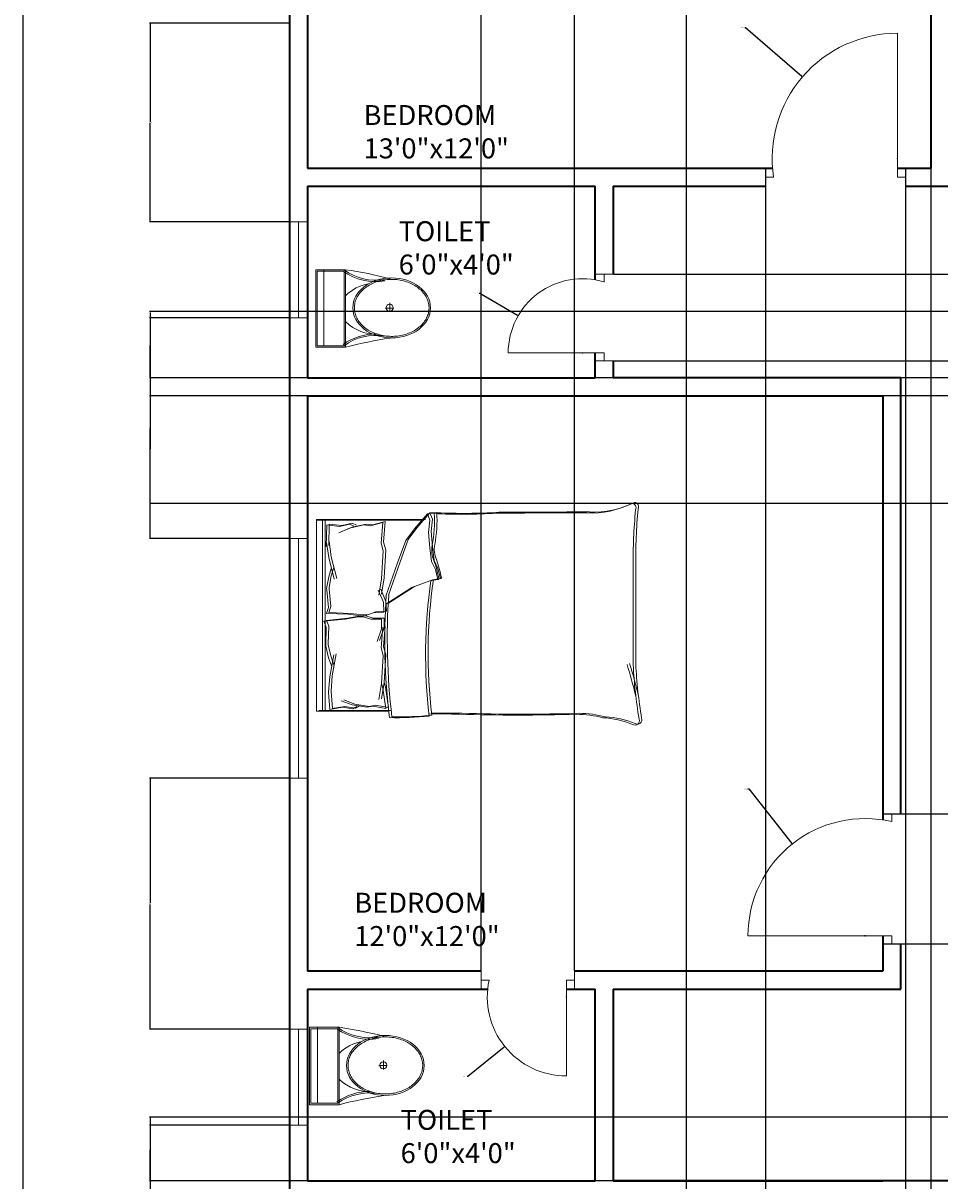
# Model space of a CAD drawing. Units: inches. Extents: x 1861 to 2564, y 1482 to 2317.
# Tile 4 of 11: x 1861 to 2090, y 1853 to 2143. Entities that reach past the tile are written whole.
import ezdxf

# ---------------------------------------------------------------- set-up
doc = ezdxf.new("R2010")
doc.units = ezdxf.units.IN
for name, color, linetype, lineweight in [('A-ANNO-DIMS', 2, 'Continuous', 18), ('A-ANNO-TTLB', 7, 'Continuous', 25), ('A-AREA-IDEN', 7, 'Continuous', 18), ('A-DOOR', 3, 'Continuous', 18), ('A-FLOR-FIXT', 8, 'Continuous', 18), ('A-FURN', 8, 'Continuous', 13), ('A-GLAZ', 4, 'Continuous', 18), ('A-WALL', 7, 'Continuous', 35)]:
    doc.layers.add(name, color=color, linetype=linetype, lineweight=lineweight)
doc.styles.get("Standard").update_dxf_attribs({"font": 'arial.ttf'})
doc.dimstyles.get("Standard").update_dxf_attribs({"dimtxt": 0.18, "dimasz": 0.18, "dimexe": 0.18, "dimexo": 0.0625, "dimgap": 0.09, "dimtad": 0, "dimtih": 1, "dimtoh": 1, "dimdec": 4, "dimzin": 0, "dimdsep": 46, "dimtxsty": 'Standard', "dimcen": 0.09, "dimadec": 0, "dimazin": 0, "dimtfac": 1, "dimtdec": 4, "dimtofl": 0, "dimtmove": 0, "dimatfit": 3, "dimfxl": 1, "dimtolj": 1, "dimtzin": 0, "dimarcsym": 0})

# ---------------------------------------------------------------- blocks, each defined once
blk = doc.blocks.new('A$C31115884')
for p, q in [((283.1, 497.7), (223.4, 497.7)), ((257.5, 466.4), (257.5, 523.2)), ((0, 200), (0, 0)), ((520, 200), (0, 200)), ((10, 190), (10, 10)), ((510, 190), (10, 190)), ((510, 10), (510, 190)), ((520, 0), (520, 200)), ((510, 54.5), (0, 54.5)), ((10, 10), (510, 10)), ((0, 0), (520, 0))]:
    blk.add_line(p, q)
blk.add_circle((255.6, 496.4), 23.6)
for centre, radius, start, end in [((2777.7, -204.6), 2807, 165.4549, 171.71327), ((3237, 905), 2807, 188.28673, 194.5451), ((-294.5, 403.3), 364.7, 324.20913, 9.34987), ((-294.5, 403.3), 374.7, 324.20913, 9.34987), ((139.5, 406.2), 293.5, 315.84364, 2.65635), ((805.8, 403.3), 374.7, 179.20365, 215.79087), ((805.8, 403.3), 364.7, 170.65013, 215.79087), ((383.6, 406.2), 293.5, 190.27735, 224.15636)]:
    blk.add_arc(centre, radius, start, end)
blk.add_ellipse((256.2, 509.9), major_axis=(0, -260.7), ratio=0.772727)
blk.add_open_spline([(256.2, 259.2), (263.1, 259.2), (270, 259.7), (287.8, 262.3), (298.7, 265.1), (319.9, 273.1), (330.2, 278.4), (350.1, 291.1), (359.7, 298.7), (377.7, 315.9), (386.2, 325.5), (401.7, 346.6), (408.8, 358.1), (421.3, 382.5), (426.8, 395.5), (435.9, 422.4), (439.5, 436.4), (444.8, 465.1), (446.5, 479.7), (447.9, 509.2), (447.6, 524), (445, 553.3), (442.7, 567.8), (436.3, 596), (432.1, 609.7), (421.9, 636), (416, 648.6), (402.5, 672.1), (395, 683), (378.6, 703), (369.8, 712.1), (351.1, 728), (341.3, 734.8), (320.9, 746.2), (310.4, 750.7), (288.9, 757.3), (278, 759.4), (256, 761), (245, 760.6), (223.1, 757.2), (212.3, 754.3), (191.1, 746.1), (180.8, 740.7), (160.9, 727.8), (151.4, 720.1), (133.5, 702.7), (125.1, 693), (109.6, 671.7), (102.6, 660.2), (90.2, 635.7), (84.9, 622.7), (76, 595.6), (72.4, 581.6), (67.2, 552.9), (65.6, 538.2), (64.4, 508.8), (64.8, 494), (67.5, 464.7), (69.9, 450.2), (76.6, 422), (80.8, 408.3), (91.1, 382.2), (97.2, 369.7), (110.8, 346.3), (118.4, 335.4), (134.8, 315.6), (143.7, 306.7), (162.4, 290.9), (172.3, 284.2), (192.8, 273), (203.3, 268.6), (224.8, 262.2), (235.8, 260.2), (249.9, 259.3), (253, 259.2), (256.2, 259.2)], degree=3, knots=[0, 0, 0, 0, 0.110105, 0.110105, 0.285049, 0.285049, 0.459994, 0.459994, 0.634938, 0.634938, 0.809882, 0.809882, 0.984827, 0.984827, 1.159771, 1.159771, 1.334715, 1.334715, 1.50966, 1.50966, 1.684604, 1.684604, 1.859549, 1.859549, 2.034493, 2.034493, 2.209437, 2.209437, 2.384382, 2.384382, 2.559326, 2.559326, 2.73427, 2.73427, 2.909215, 2.909215, 3.084159, 3.084159, 3.259103, 3.259103, 3.434048, 3.434048, 3.608992, 3.608992, 3.783936, 3.783936, 3.958881, 3.958881, 4.133825, 4.133825, 4.30877, 4.30877, 4.483714, 4.483714, 4.658658, 4.658658, 4.833603, 4.833603, 5.008547, 5.008547, 5.183491, 5.183491, 5.358436, 5.358436, 5.53338, 5.53338, 5.708324, 5.708324, 5.883269, 5.883269, 6.058213, 6.058213, 6.233158, 6.233158, 6.283185, 6.283185, 6.283185, 6.283185])
blk = doc.blocks.new('WIN-24IN')
for p, q in [((0, 24), (4.5, 24)), ((4.5, 24), (2.25, 24)), ((2.25, 24), (2.25, 0)), ((2.25, 0), (0, 0)), ((0, 0), (4.5, 0))]:
    blk.add_line(p, q)
blk = doc.blocks.new('BED-DOUBLE')
for p, q in [((3.48, 63.34), (3.48, 81.45)), ((3.48, 63.34), (3.48, 81.45)), ((51.27, 81.45), (3.48, 81.45)), ((51.27, 81.45), (51.27, 54.84)), ((51.27, 81.45), (51.27, 54.84)), ((51.27, 81.45), (51.49, 81.45)), ((51.49, 81.45), (51.49, 80.81)), ((3.48, 79.91), (51.27, 79.91)), ((3.48, 79.91), (51.27, 79.91)), ((3.7, 62.7), (3.7, 80.81)), ((3.7, 62.7), (3.7, 80.81)), ((3.7, 79.27), (51.49, 79.27)), ((3.7, 79.27), (51.49, 79.27)), ((3.9, 78.11), (8.18, 78.44)), ((3.9, 78.11), (8.18, 78.44)), ((8.18, 78.44), (8.29, 78.42)), ((8.18, 78.44), (8.29, 78.42)), ((8.29, 78.42), (12.11, 78.13)), ((8.29, 78.42), (12.11, 78.13)), ((14.86, 77.7), (16.88, 78.42)), ((14.86, 77.7), (16.88, 78.42)), ((16.88, 78.42), (19.77, 79.14)), ((16.88, 78.42), (19.77, 79.14)), ((17.11, 77.78), (20, 78.5)), ((17.11, 77.78), (20, 78.5)), ((19.77, 79.14), (20.09, 79.14)), ((19.77, 79.14), (20.09, 79.14)), ((20, 78.5), (20.32, 78.5)), ((20, 78.5), (20.32, 78.5)), ((20.09, 79.14), (24.54, 79)), ((20.09, 79.14), (24.54, 79)), ((20.32, 78.5), (24.77, 78.36)), ((20.32, 78.5), (24.77, 78.36)), ((24.54, 79), (25.98, 79.58)), ((24.54, 79), (25.98, 79.58)), ((24.77, 78.36), (26.21, 78.94)), ((24.77, 78.36), (26.21, 78.94)), ((25.98, 79.58), (26.56, 74.23)), ((25.98, 79.58), (26.56, 74.23)), ((26.21, 78.94), (26.79, 73.59)), ((26.21, 78.94), (26.79, 73.59)), ((27.98, 78.95), (27.73, 73.58)), ((27.98, 78.95), (27.73, 73.58)), ((28.21, 78.31), (27.96, 72.94)), ((28.21, 78.31), (27.96, 72.94)), ((29.46, 78.47), (27.98, 78.95)), ((29.46, 78.47), (27.98, 78.95)), ((29.69, 77.83), (28.21, 78.31)), ((29.68, 77.83), (28.21, 78.31)), ((33.88, 78.89), (29.46, 78.47)), ((33.88, 78.89), (29.46, 78.47)), ((34.11, 78.25), (29.68, 77.83)), ((34.11, 78.25), (29.69, 77.83)), ((34.21, 78.91), (33.88, 78.89)), ((34.21, 78.91), (33.88, 78.89)), ((34.43, 78.27), (34.11, 78.25)), ((34.43, 78.27), (34.11, 78.25)), ((37.14, 78.37), (34.21, 78.91)), ((37.14, 78.37), (34.21, 78.91)), ((37.36, 77.73), (34.43, 78.27)), ((37.36, 77.73), (34.43, 78.27)), ((41.92, 78.38), (36.5, 77.02)), ((41.92, 78.38), (36.5, 77.02)), ((39.2, 77.77), (37.14, 78.37)), ((39.2, 77.77), (37.14, 78.37)), ((45.71, 78.9), (41.92, 78.38)), ((45.71, 78.9), (41.92, 78.38)), ((45.94, 78.26), (42.14, 77.74)), ((45.94, 78.26), (42.14, 77.74)), ((50.11, 78.89), (44.71, 78.99)), ((44.71, 78.99), (45.71, 78.9)), ((50.11, 78.89), (44.71, 78.99)), ((44.71, 78.99), (45.71, 78.9)), ((50.34, 78.25), (44.94, 78.35)), ((44.94, 78.35), (45.94, 78.26)), ((50.34, 78.25), (44.94, 78.35)), ((44.94, 78.35), (45.94, 78.26)), ((50.11, 78.89), (49.73, 75.68)), ((50.11, 78.89), (49.73, 75.68)), ((50.34, 78.25), (49.96, 75.04)), ((50.34, 78.25), (49.96, 75.04)), ((51.49, 80.81), (51.49, 54.2)), ((51.49, 80.81), (51.49, 54.2)), ((3.9, 78.13), (4.47, 74.95)), ((3.9, 78.13), (4.47, 74.95)), ((4.12, 77.49), (4.7, 74.31)), ((4.12, 77.49), (4.7, 74.31)), ((4.13, 77.47), (8.41, 77.8)), ((4.13, 77.47), (8.41, 77.8)), ((8.41, 77.8), (8.51, 77.78)), ((8.41, 77.8), (8.51, 77.78)), ((8.51, 77.78), (12.34, 77.49)), ((8.51, 77.78), (12.34, 77.49)), ((12.11, 78.13), (17.6, 77.12)), ((12.11, 78.13), (17.6, 77.12)), ((12.34, 77.49), (17.83, 76.48)), ((12.34, 77.49), (17.83, 76.48)), ((15.08, 77.06), (17.11, 77.78)), ((15.08, 77.06), (17.11, 77.78)), ((42.14, 77.74), (36.72, 76.38)), ((42.14, 77.74), (36.72, 76.38)), ((39.43, 77.13), (37.36, 77.73)), ((39.43, 77.13), (37.36, 77.73)), ((49.31, 73.19), (48.13, 75.87)), ((49.31, 73.19), (48.13, 75.87)), ((49.73, 75.68), (50.33, 73.11)), ((49.73, 75.68), (50.33, 73.11)), ((4.47, 74.95), (4.04, 72.35)), ((4.47, 74.95), (4.04, 72.35)), ((4.7, 74.31), (4.27, 71.71)), ((4.7, 74.31), (4.27, 71.71)), ((4.47, 68.88), (5.05, 72.49)), ((4.47, 68.88), (5.05, 72.49)), ((5.05, 72.49), (6.06, 75.24)), ((5.05, 72.49), (6.06, 75.24)), ((5.28, 71.85), (6.29, 74.6)), ((5.28, 71.85), (6.29, 74.6)), ((26.56, 74.23), (27.14, 71.04)), ((26.56, 74.23), (27.14, 71.04)), ((26.79, 73.59), (27.37, 70.41)), ((26.79, 73.59), (27.37, 70.41)), ((27.73, 73.58), (27.36, 70.37)), ((27.73, 73.58), (27.36, 70.37)), ((27.96, 72.94), (27.58, 69.73)), ((27.96, 72.94), (27.58, 69.73)), ((49.54, 72.55), (48.36, 75.23)), ((49.54, 72.55), (48.36, 75.23)), ((50.11, 69.62), (49.31, 73.19)), ((50.11, 69.62), (49.31, 73.19)), ((50.34, 68.98), (49.54, 72.55)), ((50.34, 68.98), (49.54, 72.55)), ((50.33, 73.11), (49.82, 72.06)), ((50.33, 73.11), (49.82, 72.06)), ((49.96, 75.04), (50.56, 72.47)), ((49.96, 75.04), (50.56, 72.47)), ((50.56, 72.47), (50.04, 71.42)), ((50.56, 72.47), (50.04, 71.42)), ((4.04, 72.35), (4.62, 71.33)), ((4.04, 72.35), (4.62, 71.33)), ((4.27, 71.71), (4.85, 70.69)), ((4.27, 71.71), (4.85, 70.69)), ((4.7, 68.24), (5.28, 71.85)), ((4.7, 68.24), (5.28, 71.85)), ((27.14, 69.74), (26.56, 67.86)), ((27.14, 69.74), (26.56, 67.86)), ((27.14, 71.04), (27.14, 69.74)), ((27.14, 71.04), (27.14, 69.74)), ((27.36, 70.37), (27.44, 69.07)), ((27.36, 70.37), (27.44, 69.07)), ((27.37, 70.41), (27.37, 69.1)), ((27.37, 70.41), (27.37, 69.1)), ((27.58, 69.73), (27.67, 68.43)), ((27.58, 69.73), (27.67, 68.43)), ((49.92, 68.01), (50.11, 69.62)), ((49.92, 68.01), (50.11, 69.62)), ((4.18, 64.1), (4.76, 67.29)), ((4.18, 64.1), (4.76, 67.29)), ((4.76, 67.29), (4.47, 68.88)), ((4.76, 67.29), (4.47, 68.88)), ((4.99, 66.65), (4.7, 68.24)), ((4.99, 66.65), (4.7, 68.24)), ((26.56, 67.86), (26.56, 65.18)), ((26.56, 67.86), (26.56, 65.18)), ((27.37, 69.1), (26.79, 67.22)), ((27.37, 69.1), (26.79, 67.22)), ((26.79, 67.22), (26.79, 64.54)), ((26.79, 67.22), (26.79, 64.54)), ((27.44, 69.07), (28.13, 67.23)), ((27.44, 69.07), (28.13, 67.23)), ((27.67, 68.43), (28.36, 66.59)), ((27.67, 68.43), (28.36, 66.59)), ((28.13, 67.23), (28.3, 64.55)), ((28.13, 67.23), (28.3, 64.55)), ((50.7, 64.87), (49.92, 68.01)), ((50.7, 64.87), (49.92, 68.01)), ((50.15, 67.37), (50.34, 68.98)), ((50.15, 67.37), (50.34, 68.98)), ((50.93, 64.23), (50.15, 67.37)), ((50.93, 64.23), (50.15, 67.37)), ((9.28, 64.83), (4.18, 64.1)), ((9.28, 64.83), (4.18, 64.1)), ((4.41, 63.46), (4.99, 66.65)), ((4.41, 63.46), (4.99, 66.65)), ((9.51, 64.19), (4.41, 63.46)), ((9.51, 64.19), (4.41, 63.46)), ((6.38, 65.82), (10.41, 65.15)), ((6.38, 65.82), (10.41, 65.15)), ((6.61, 65.18), (10.64, 64.51)), ((6.61, 65.18), (10.64, 64.51)), ((10.41, 65.15), (9.28, 64.83)), ((10.41, 65.15), (9.28, 64.83)), ((10.64, 64.51), (9.51, 64.19)), ((10.64, 64.51), (9.51, 64.19)), ((10.41, 65.15), (17.42, 64.72)), ((10.41, 65.15), (17.42, 64.72)), ((10.64, 64.51), (17.65, 64.08)), ((10.64, 64.51), (17.65, 64.08)), ((17.42, 64.72), (19.38, 65.28)), ((17.42, 64.72), (19.38, 65.28)), ((17.65, 64.08), (19.61, 64.64)), ((17.65, 64.08), (19.61, 64.64)), ((19.38, 65.28), (24.52, 64.87)), ((19.38, 65.28), (24.52, 64.87)), ((19.61, 64.64), (24.75, 64.23)), ((19.61, 64.64), (24.74, 64.23)), ((24.1, 65.18), (20.96, 66.27)), ((24.1, 65.18), (20.96, 66.27)), ((24.33, 64.54), (21.19, 65.63)), ((24.33, 64.54), (21.19, 65.63)), ((26.56, 65.18), (24.1, 65.18)), ((26.56, 65.18), (24.1, 65.18)), ((26.79, 64.54), (24.33, 64.54)), ((26.79, 64.54), (24.33, 64.54)), ((28.3, 64.55), (30.75, 64.71)), ((28.3, 64.55), (30.75, 64.71)), ((28.36, 66.59), (28.53, 63.91)), ((28.36, 66.59), (28.53, 63.91)), ((28.53, 63.91), (30.98, 64.07)), ((28.53, 63.91), (30.98, 64.07)), ((30.26, 64.06), (34.45, 57.57)), ((30.26, 64.06), (34.45, 57.57)), ((30.75, 64.71), (33.82, 65.99)), ((30.75, 64.71), (33.82, 65.99)), ((30.98, 64.07), (34.05, 65.35)), ((30.98, 64.07), (34.05, 65.35)), ((40.65, 61.13), (32.31, 64.06)), ((40.64, 61.13), (32.31, 64.06)), ((32.56, 65.82), (36.6, 65.15)), ((32.57, 65.82), (36.6, 65.15)), ((32.79, 65.18), (36.83, 64.51)), ((32.79, 65.18), (36.83, 64.51)), ((36.6, 65.15), (43.61, 64.72)), ((36.6, 65.15), (43.61, 64.72)), ((36.83, 64.51), (43.84, 64.08)), ((36.83, 64.51), (43.84, 64.08)), ((43.61, 64.72), (45.57, 65.28)), ((43.61, 64.72), (45.57, 65.28)), ((43.84, 64.08), (45.8, 64.64)), ((43.84, 64.08), (45.8, 64.64)), ((45.57, 65.28), (50.7, 64.87)), ((45.57, 65.28), (50.7, 64.87)), ((45.8, 64.64), (50.93, 64.23)), ((45.8, 64.64), (50.93, 64.23)), ((30.49, 63.42), (34.68, 56.93)), ((30.49, 63.42), (34.68, 56.93)), ((40.87, 60.49), (32.54, 63.42)), ((40.87, 60.49), (32.54, 63.42)), ((46.22, 59.12), (40.64, 61.13)), ((46.22, 59.12), (40.65, 61.13)), ((46.45, 58.48), (40.87, 60.49)), ((46.45, 58.48), (40.87, 60.49)), ((49.16, 56.95), (46.22, 59.12)), ((49.16, 56.95), (46.22, 59.12)), ((49.39, 56.31), (46.45, 58.48)), ((49.39, 56.31), (46.45, 58.48)), ((34.45, 57.57), (36.15, 53.08)), ((34.45, 57.57), (36.15, 53.08)), ((34.68, 56.93), (36.38, 52.44)), ((34.68, 56.93), (36.38, 52.44)), ((52.87, 53.7), (49.16, 56.95)), ((52.87, 53.7), (49.16, 56.95)), ((53.1, 53.06), (49.39, 56.31)), ((53.1, 53.06), (49.39, 56.31)), ((36.15, 53.08), (36.46, 51.07)), ((36.15, 53.08), (36.46, 51.07)), ((36.38, 52.44), (36.69, 50.43)), ((36.38, 52.44), (36.69, 50.43)), ((38.94, 51.69), (40.95, 52.62)), ((38.94, 51.69), (40.95, 52.62)), ((40.95, 52.62), (44.36, 53.08)), ((40.95, 52.62), (44.36, 53.08)), ((41.18, 51.98), (44.59, 52.44)), ((41.18, 51.98), (44.59, 52.44)), ((44.36, 53.08), (48.23, 53.39)), ((44.36, 53.08), (48.23, 53.39)), ((44.59, 52.44), (48.46, 52.75)), ((44.59, 52.44), (48.46, 52.75)), ((48.23, 53.39), (51.33, 53.08)), ((48.23, 53.39), (51.33, 53.08)), ((48.46, 52.75), (51.56, 52.44)), ((48.46, 52.75), (51.56, 52.44)), ((51.33, 53.08), (52.87, 53.7)), ((51.33, 53.08), (52.87, 53.7)), ((51.56, 52.44), (53.1, 53.06)), ((51.56, 52.44), (53.1, 53.06)), ((52.95, 51.95), (52.87, 53.7, 3.87)), ((52.95, 51.95), (52.87, 53.7, 3.87)), ((53.18, 51.32), (53.1, 53.06, 3.87)), ((53.18, 51.32), (53.1, 53.06, 3.87)), ((36.46, 51.07), (38.94, 51.69)), ((36.46, 51.07), (38.94, 51.69)), ((36.69, 50.43), (39.17, 51.05)), ((36.69, 50.43), (39.17, 51.05)), ((39.17, 51.05), (41.18, 51.98)), ((39.17, 51.05), (41.18, 51.98)), ((15.06, 2.2), (39.68, 2.2)), ((15.06, 2.2), (39.68, 2.2)), ((15.29, 1.56), (39.91, 1.56)), ((15.29, 1.56), (39.91, 1.56))]:
    blk.add_line(p, q)
for centre, radius, start, end in [((21.36, -100.61), 164.97, 86.0865, 96.7821), ((21.36, -100.61), 164.97, 86.0865, 96.7821), ((85.16, 61.35), 83.31, 178.7218, 185.604), ((85.16, 61.35), 83.31, 178.7218, 185.604), ((85.39, 60.71), 83.31, 178.7218, 185.604), ((85.39, 60.71), 83.31, 178.7218, 185.604), ((21.59, -101.25), 164.97, 86.0865, 96.7821), ((21.59, -101.25), 164.97, 86.0865, 96.7821), ((17.76, -74.87), 129.02, 81.7845, 96.9006), ((17.76, -74.87), 129.02, 81.7845, 96.9006), ((17.99, -75.51), 129.02, 81.7845, 96.9006), ((17.98, -75.51), 129.02, 81.7845, 96.9006), ((-167.31, 50.27), 170.11, 358.4762, 1.0082), ((-167.31, 50.27), 170.11, 358.4762, 1.0082), ((-167.08, 49.63), 170.11, 358.4762, 1.0082), ((-167.08, 49.63), 170.11, 358.4762, 1.0082), ((43.74, 46.38), 6.22, 78.6608, 113.7384), ((43.74, 46.38), 6.22, 78.6608, 113.7384), ((51.33, 88.1), 36.18, 259.8763, 272.5657), ((51.33, 88.1), 36.18, 259.8763, 272.5657), ((36.64, 51.01), 0.185, 160.2464, 271.1377), ((36.64, 51.01), 0.185, 160.2464, 271.1377), ((31.15, 79.96), 29.65, 280.6617, 289.8806), ((31.15, 79.96), 29.65, 280.6617, 289.8806), ((36.87, 50.37), 0.185, 160.2464, 271.1377), ((36.87, 50.37), 0.185, 160.2464, 271.1377), ((31.38, 79.32), 29.65, 280.6617, 289.8806), ((31.38, 79.32), 29.65, 280.6617, 289.8806), ((43.97, 45.74), 6.22, 78.6608, 113.7384), ((43.97, 45.74), 6.22, 78.6608, 113.7384), ((51.56, 87.46), 36.18, 259.8763, 272.5657), ((51.56, 87.46), 36.18, 259.8763, 272.5657), ((182.27, 45.13), 129.5, 176.9791, 183.8365), ((182.27, 45.13), 129.5, 176.9791, 183.8365), ((182.5, 44.49), 129.5, 176.9791, 183.8365), ((182.49, 44.49), 129.5, 176.9791, 183.8365), ((484.82, 30.83), 482.31, 178.2277, 181.7185), ((484.82, 30.83), 482.31, 178.2277, 181.7185), ((485.05, 30.19), 482.31, 178.2277, 181.7185), ((485.05, 30.19), 482.31, 178.2277, 181.7185), ((-4508.74, 13.62), 4561.86, 0.00217, 0.28689), ((-4508.74, 13.62), 4561.86, 0.00217, 0.28689), ((-4508.51, 12.98), 4561.86, 0.00217, 0.28689), ((-4508.51, 12.98), 4561.86, 0.00217, 0.28689), ((-26.9, 16.93), 29.63, 346.0648, 358.9113), ((-26.9, 16.93), 29.63, 346.0648, 358.9113), ((-26.67, 16.29), 29.63, 346.0648, 358.9113), ((-26.67, 16.29), 29.63, 346.0648, 358.9113), ((76.16, 12.78), 23.07, 177.4714, 206.4681), ((76.16, 12.78), 23.07, 177.4714, 206.4681), ((76.39, 12.14), 23.07, 177.4714, 206.4681), ((76.39, 12.14), 23.07, 177.4714, 206.4681), ((-21.66, 11.17), 23.56, 337.9751, 356.652), ((-21.66, 11.17), 23.56, 337.9751, 356.652), ((-21.43, 10.53), 23.56, 337.9751, 356.652), ((-21.43, 10.53), 23.56, 337.9751, 356.652), ((-17.22, 105.16), 106.46, 283.3832, 287.7053), ((-17.22, 105.16), 106.46, 283.3832, 287.7053), ((-16.99, 104.52), 106.46, 283.3832, 287.7053), ((-16.99, 104.52), 106.46, 283.3832, 287.7053), ((1.09, 1.73), 1.09, 146.1736, 293.4781), ((1.09, 1.73), 1.09, 146.1736, 293.4781), ((1.32, 1.09), 1.09, 146.1736, 293.4781), ((1.32, 1.09), 1.09, 146.1736, 293.4781), ((21.43, -119.39), 121.76, 92.9958, 99.4091), ((21.43, -119.39), 121.76, 92.9958, 99.4091), ((21.66, -120.03), 121.76, 92.9958, 99.4091), ((21.66, -120.03), 121.76, 92.9958, 99.4091), ((41.15, -130.83), 133.04, 84.4998, 90.6351), ((41.15, -130.83), 133.04, 84.4998, 90.6351), ((41.38, -131.47), 133.04, 84.4998, 90.6351), ((41.38, -131.47), 133.04, 84.4998, 90.6351), ((54.41, 2.58), 1.1, 242.6588, 356.02), ((54.41, 2.58), 1.1, 242.6588, 356.02), ((54.64, 1.94), 1.1, 242.6588, 356.02), ((54.64, 1.94), 1.1, 242.6588, 356.02)]:
    blk.add_arc(centre, radius, start, end)
blk = doc.blocks.new('*D35')
at = {"layer": 'A-ANNO-DIMS', "color": 0, "lineweight": -2, "transparency": 16777216}
for p, q in [((2026.99, 2250.82), (2026.99, 1545.6)), ((2088.24, 2250.82), (2088.24, 1545.6)), ((2027.17, 1545.78), (2057.22, 1545.78)), ((2088.06, 1545.78), (2058.01, 1545.78))]:
    blk.add_line(p, q, dxfattribs=at)
at = {"layer": 'A-ANNO-DIMS', "color": 0, "transparency": 16777216}
for points in [[(2027.17, 1545.81), (2027.17, 1545.75), (2026.99, 1545.78)], [(2088.06, 1545.81), (2088.06, 1545.75), (2088.24, 1545.78)]]:
    blk.add_solid(points, dxfattribs=at)
at = {"layer": 'Defpoints', "color": 0, "transparency": 16777216}
for p in [(2026.99, 2250.89), (2088.24, 2250.89), (2088.24, 1545.78)]:
    blk.add_point(p, dxfattribs=at)
at = {"layer": 'A-ANNO-DIMS', "color": 0, "transparency": 16777216, "insert": (2057.61, 1545.78), "char_height": 0.18, "attachment_point": 5}
blk.add_mtext('\\A1;61.25', dxfattribs=at)
blk = doc.blocks.new('*D40')
at = {"layer": 'A-ANNO-DIMS', "color": 0, "lineweight": -2, "transparency": 16777216}
for p, q in [((1927.68, 2143.17), (1892.76, 2143.17)), ((1892.94, 2142.99), (1892.94, 2118.48)), ((1892.94, 2093.61), (1892.94, 2118.12)), ((1927.68, 2093.43), (1892.76, 2093.43))]:
    blk.add_line(p, q, dxfattribs=at)
at = {"layer": 'A-ANNO-DIMS', "color": 0, "transparency": 16777216}
for points in [[(1892.91, 2142.99), (1892.97, 2142.99), (1892.94, 2143.17)], [(1892.91, 2093.61), (1892.97, 2093.61), (1892.94, 2093.43)]]:
    blk.add_solid(points, dxfattribs=at)
at = {"layer": 'Defpoints', "color": 0, "transparency": 16777216}
for p in [(1927.74, 2143.17), (1892.94, 2093.43), (1927.74, 2093.43)]:
    blk.add_point(p, dxfattribs=at)
at = {"layer": 'A-ANNO-DIMS', "color": 0, "transparency": 16777216, "insert": (1892.94, 2118.3), "char_height": 0.18, "attachment_point": 5}
blk.add_mtext('\\A1;49.73', dxfattribs=at)
blk = doc.blocks.new('*D41')
at = {"layer": 'A-ANNO-DIMS', "color": 0, "lineweight": -2, "transparency": 16777216}
for p, q in [((1927.68, 2069.43), (1892.76, 2069.43)), ((1892.94, 2069.25), (1892.94, 2042)), ((1892.94, 2014.38), (1892.94, 2041.64)), ((1927.68, 2014.2), (1892.76, 2014.2))]:
    blk.add_line(p, q, dxfattribs=at)
at = {"layer": 'A-ANNO-DIMS', "color": 0, "transparency": 16777216}
for points in [[(1892.91, 2069.25), (1892.97, 2069.25), (1892.94, 2069.43)], [(1892.91, 2014.38), (1892.97, 2014.38), (1892.94, 2014.2)]]:
    blk.add_solid(points, dxfattribs=at)
at = {"layer": 'Defpoints', "color": 0, "transparency": 16777216}
for p in [(1927.74, 2069.43), (1892.94, 2014.2), (1927.74, 2014.2)]:
    blk.add_point(p, dxfattribs=at)
at = {"layer": 'A-ANNO-DIMS', "color": 0, "transparency": 16777216, "insert": (1892.94, 2041.82), "char_height": 0.18, "attachment_point": 5}
blk.add_mtext('\\A1;55.23', dxfattribs=at)
blk = doc.blocks.new('*D42')
at = {"layer": 'A-ANNO-DIMS', "color": 0, "lineweight": -2, "transparency": 16777216}
for p, q in [((1927.68, 1954.2), (1892.76, 1954.2)), ((1892.94, 1954.02), (1892.94, 1922.95)), ((1892.94, 1891.51), (1892.94, 1922.58)), ((1927.68, 1891.33), (1892.76, 1891.33))]:
    blk.add_line(p, q, dxfattribs=at)
at = {"layer": 'A-ANNO-DIMS', "color": 0, "transparency": 16777216}
for points in [[(1892.91, 1954.02), (1892.97, 1954.02), (1892.94, 1954.2)], [(1892.91, 1891.51), (1892.97, 1891.51), (1892.94, 1891.33)]]:
    blk.add_solid(points, dxfattribs=at)
at = {"layer": 'Defpoints', "color": 0, "transparency": 16777216}
for p in [(1927.74, 1954.2), (1892.94, 1891.33), (1927.74, 1891.33)]:
    blk.add_point(p, dxfattribs=at)
at = {"layer": 'A-ANNO-DIMS', "color": 0, "transparency": 16777216, "insert": (1892.94, 1922.76), "char_height": 0.18, "attachment_point": 5}
blk.add_mtext('\\A1;62.88', dxfattribs=at)
blk = doc.blocks.new('*D43')
at = {"layer": 'A-ANNO-DIMS', "color": 0, "lineweight": -2, "transparency": 16777216}
for p, q in [((1927.68, 1867.33), (1892.76, 1867.33)), ((1892.94, 1867.15), (1892.94, 1820.91)), ((1892.94, 1774.31), (1892.94, 1820.55)), ((1927.68, 1774.13), (1892.76, 1774.13))]:
    blk.add_line(p, q, dxfattribs=at)
at = {"layer": 'A-ANNO-DIMS', "color": 0, "transparency": 16777216}
for points in [[(1892.91, 1867.15), (1892.97, 1867.15), (1892.94, 1867.33)], [(1892.91, 1774.31), (1892.97, 1774.31), (1892.94, 1774.13)]]:
    blk.add_solid(points, dxfattribs=at)
at = {"layer": 'Defpoints', "color": 0, "transparency": 16777216}
for p in [(1927.74, 1867.33), (1892.94, 1774.13), (1927.74, 1774.13)]:
    blk.add_point(p, dxfattribs=at)
at = {"layer": 'A-ANNO-DIMS', "color": 0, "transparency": 16777216, "insert": (1892.94, 1820.73), "char_height": 0.18, "attachment_point": 5}
blk.add_mtext('\\A1;93.19', dxfattribs=at)
blk = doc.blocks.new('*D51')
at = {"layer": 'A-ANNO-DIMS', "color": 0, "lineweight": -2, "transparency": 16777216}
for p, q in [((2046.87, 2106.82), (2046.87, 1545.6)), ((2081.9, 2106.82), (2081.9, 1545.6)), ((2047.05, 1545.78), (2063.92, 1545.78)), ((2081.72, 1545.78), (2064.85, 1545.78))]:
    blk.add_line(p, q, dxfattribs=at)
at = {"layer": 'A-ANNO-DIMS', "color": 0, "transparency": 16777216}
for points in [[(2047.05, 1545.81), (2047.05, 1545.75), (2046.87, 1545.78)], [(2081.72, 1545.81), (2081.72, 1545.75), (2081.9, 1545.78)]]:
    blk.add_solid(points, dxfattribs=at)
at = {"layer": 'Defpoints', "color": 0, "transparency": 16777216}
for p in [(2046.87, 2106.89), (2081.9, 2106.89), (2081.9, 1545.78)]:
    blk.add_point(p, dxfattribs=at)
at = {"layer": 'A-ANNO-DIMS', "color": 0, "transparency": 16777216, "insert": (2064.39, 1545.78), "char_height": 0.18, "attachment_point": 5}
blk.add_mtext('\\A1;35.035', dxfattribs=at)
blk = doc.blocks.new('*D53')
at = {"layer": 'A-ANNO-DIMS', "color": 0, "lineweight": -2, "transparency": 16777216}
for p, q in [((2076.3, 1945.29), (2537.22, 1945.29)), ((2537.04, 1945.11), (2537.04, 1929.2)), ((2537.04, 1912.93), (2537.04, 1928.84)), ((2076.3, 1912.75), (2537.22, 1912.75))]:
    blk.add_line(p, q, dxfattribs=at)
at = {"layer": 'A-ANNO-DIMS', "color": 0, "transparency": 16777216}
for points in [[(2537.01, 1945.11), (2537.07, 1945.11), (2537.04, 1945.29)], [(2537.01, 1912.93), (2537.07, 1912.93), (2537.04, 1912.75)]]:
    blk.add_solid(points, dxfattribs=at)
at = {"layer": 'Defpoints', "color": 0, "transparency": 16777216}
for p in [(2076.24, 1945.29), (2537.04, 1945.29), (2076.24, 1912.75)]:
    blk.add_point(p, dxfattribs=at)
at = {"layer": 'A-ANNO-DIMS', "color": 0, "transparency": 16777216, "insert": (2537.04, 1929.02), "char_height": 0.18, "attachment_point": 5}
blk.add_mtext('\\A1;32.544', dxfattribs=at)
blk = doc.blocks.new('*D54')
at = {"layer": 'A-ANNO-DIMS', "color": 0, "lineweight": -2, "transparency": 16777216}
for p, q in [((1975.71, 1905.95), (1975.71, 2290.37)), ((1975.89, 2290.19), (1986.91, 2290.19)), ((1998.87, 2290.19), (1987.85, 2290.19)), ((1999.05, 1905.95), (1999.05, 2290.37))]:
    blk.add_line(p, q, dxfattribs=at)
at = {"layer": 'A-ANNO-DIMS', "color": 0, "transparency": 16777216}
for points in [[(1975.89, 2290.22), (1975.89, 2290.16), (1975.71, 2290.19)], [(1998.87, 2290.22), (1998.87, 2290.16), (1999.05, 2290.19)]]:
    blk.add_solid(points, dxfattribs=at)
at = {"layer": 'Defpoints', "color": 0, "transparency": 16777216}
for p in [(1999.05, 2290.19), (1975.71, 1905.89), (1999.05, 1905.89)]:
    blk.add_point(p, dxfattribs=at)
at = {"layer": 'A-ANNO-DIMS', "color": 0, "transparency": 16777216, "insert": (1987.38, 2290.19), "char_height": 0.18, "attachment_point": 5}
blk.add_mtext('\\A1;23.335', dxfattribs=at)
blk = doc.blocks.new('*D61')
at = {"layer": 'A-ANNO-DIMS', "color": 0, "lineweight": -2, "transparency": 16777216}
for p, q in [((2008.8, 2080.33), (2537.22, 2080.33)), ((2537.04, 2080.15), (2537.04, 2069.66)), ((2537.04, 2058.82), (2537.04, 2069.3)), ((2008.8, 2058.64), (2537.22, 2058.64))]:
    blk.add_line(p, q, dxfattribs=at)
at = {"layer": 'A-ANNO-DIMS', "color": 0, "transparency": 16777216}
for points in [[(2537.01, 2080.15), (2537.07, 2080.15), (2537.04, 2080.33)], [(2537.01, 2058.82), (2537.07, 2058.82), (2537.04, 2058.64)]]:
    blk.add_solid(points, dxfattribs=at)
at = {"layer": 'Defpoints', "color": 0, "transparency": 16777216}
for p in [(2008.74, 2080.33), (2537.04, 2080.33), (2008.74, 2058.64)]:
    blk.add_point(p, dxfattribs=at)
at = {"layer": 'A-ANNO-DIMS', "color": 0, "transparency": 16777216, "insert": (2537.04, 2069.48), "char_height": 0.18, "attachment_point": 5}
blk.add_mtext('\\A1;21.693', dxfattribs=at)
blk = doc.blocks.new('*D64')
at = {"layer": 'A-ANNO-DIMS', "color": 0, "lineweight": -2, "transparency": 16777216}
for p, q in [((2497.68, 2070.96), (1892.76, 2070.96)), ((1892.94, 2070.78), (1892.94, 2062.85)), ((1892.94, 2054.57), (1892.94, 2062.49)), ((2497.68, 2054.39), (1892.76, 2054.39))]:
    blk.add_line(p, q, dxfattribs=at)
at = {"layer": 'A-ANNO-DIMS', "color": 0, "transparency": 16777216}
for points in [[(1892.91, 2070.78), (1892.97, 2070.78), (1892.94, 2070.96)], [(1892.91, 2054.57), (1892.97, 2054.57), (1892.94, 2054.39)]]:
    blk.add_solid(points, dxfattribs=at)
at = {"layer": 'Defpoints', "color": 0, "transparency": 16777216}
for p in [(2497.74, 2070.96), (1892.94, 2054.39), (2497.74, 2054.39)]:
    blk.add_point(p, dxfattribs=at)
at = {"layer": 'A-ANNO-DIMS', "color": 0, "transparency": 16777216, "insert": (1892.94, 2062.67), "char_height": 0.18, "attachment_point": 5}
blk.add_mtext('\\A1;16.57', dxfattribs=at)
blk = doc.blocks.new('*D65')
at = {"layer": 'A-ANNO-DIMS', "color": 0, "lineweight": -2, "transparency": 16777216}
for p, q in [((2497.68, 2049.89), (1892.76, 2049.89)), ((1892.94, 2049.71), (1892.94, 2036.58)), ((1892.94, 2023.09), (1892.94, 2036.22)), ((2497.68, 2022.91), (1892.76, 2022.91))]:
    blk.add_line(p, q, dxfattribs=at)
at = {"layer": 'A-ANNO-DIMS', "color": 0, "transparency": 16777216}
for points in [[(1892.91, 2049.71), (1892.97, 2049.71), (1892.94, 2049.89)], [(1892.91, 2023.09), (1892.97, 2023.09), (1892.94, 2022.91)]]:
    blk.add_solid(points, dxfattribs=at)
at = {"layer": 'Defpoints', "color": 0, "transparency": 16777216}
for p in [(2497.74, 2049.89), (1892.94, 2022.91), (2497.74, 2022.91)]:
    blk.add_point(p, dxfattribs=at)
at = {"layer": 'A-ANNO-DIMS', "color": 0, "transparency": 16777216, "insert": (1892.94, 2036.4), "char_height": 0.18, "attachment_point": 5}
blk.add_mtext('\\A1;26.973', dxfattribs=at)
blk = doc.blocks.new('*D66')
at = {"layer": 'A-ANNO-DIMS', "color": 0, "lineweight": -2, "transparency": 16777216}
for p, q in [((2497.68, 1869.33), (1892.76, 1869.33)), ((1892.94, 1869.15), (1892.94, 1861.54)), ((1892.94, 1853.57), (1892.94, 1861.17)), ((2497.68, 1853.39), (1892.76, 1853.39))]:
    blk.add_line(p, q, dxfattribs=at)
at = {"layer": 'A-ANNO-DIMS', "color": 0, "transparency": 16777216}
for points in [[(1892.91, 1869.15), (1892.97, 1869.15), (1892.94, 1869.33)], [(1892.91, 1853.57), (1892.97, 1853.57), (1892.94, 1853.39)]]:
    blk.add_solid(points, dxfattribs=at)
at = {"layer": 'Defpoints', "color": 0, "transparency": 16777216}
for p in [(2497.74, 1869.33), (1892.94, 1853.39), (2497.74, 1853.39)]:
    blk.add_point(p, dxfattribs=at)
at = {"layer": 'A-ANNO-DIMS', "color": 0, "transparency": 16777216, "insert": (1892.94, 1861.36), "char_height": 0.18, "attachment_point": 5}
blk.add_mtext('\\A1;15.94', dxfattribs=at)
blk = doc.blocks.new('*D76')
at = {"layer": 'A-ANNO-DIMS', "color": 0, "lineweight": -2, "transparency": 16777216}
for p, q in [((2041.7, 2142.04), (2041.88, 2142.04)), ((2041.88, 2142.04), (2056, 2129.86)), ((2079.81, 2109.26), (2079.99, 2109.26)), ((2079.9, 2109.17), (2079.9, 2109.35))]:
    blk.add_line(p, q, dxfattribs=at)
at = {"layer": 'A-ANNO-DIMS', "color": 0, "transparency": 16777216}
blk.add_solid([(2056.02, 2129.89), (2055.98, 2129.84), (2056.14, 2129.75)], dxfattribs=at)
at = {"layer": 'Defpoints', "color": 0, "transparency": 16777216}
for p in [(2056.14, 2129.75), (2079.9, 2109.26)]:
    blk.add_point(p, dxfattribs=at)
at = {"layer": 'A-ANNO-DIMS', "color": 0, "transparency": 16777216, "insert": (2041.22, 2142.04), "char_height": 0.18, "attachment_point": 5}
blk.add_mtext('\\A1;R31.38', dxfattribs=at)
blk = doc.blocks.new('*D80')
at = {"layer": 'A-ANNO-DIMS', "color": 0, "lineweight": -2, "transparency": 16777216}
for p, q in [((2042.48, 1951.5), (2042.66, 1951.5)), ((2042.66, 1951.5), (2053.48, 1937.86)), ((2071.72, 1914.75), (2071.9, 1914.75)), ((2071.81, 1914.66), (2071.81, 1914.84))]:
    blk.add_line(p, q, dxfattribs=at)
at = {"layer": 'A-ANNO-DIMS', "color": 0, "transparency": 16777216}
blk.add_solid([(2053.5, 1937.88), (2053.46, 1937.84), (2053.59, 1937.72)], dxfattribs=at)
at = {"layer": 'Defpoints', "color": 0, "transparency": 16777216}
for p in [(2053.59, 1937.72), (2071.81, 1914.75)]:
    blk.add_point(p, dxfattribs=at)
at = {"layer": 'A-ANNO-DIMS', "color": 0, "transparency": 16777216, "insert": (2041.93, 1951.5), "char_height": 0.18, "attachment_point": 5}
blk.add_mtext('\\A1;R29.316', dxfattribs=at)
blk = doc.blocks.new('*D86')
at = {"layer": 'A-ANNO-DIMS', "color": 0, "lineweight": -2, "transparency": 16777216}
for p, q in [((1996.96, 1899.42), (1997.14, 1899.42)), ((1997.05, 1899.33), (1997.05, 1899.51)), ((1972.39, 1879.56), (1981.5, 1886.9)), ((1972.21, 1879.56), (1972.39, 1879.56))]:
    blk.add_line(p, q, dxfattribs=at)
at = {"layer": 'A-ANNO-DIMS', "color": 0, "transparency": 16777216}
blk.add_solid([(1981.48, 1886.92), (1981.52, 1886.87), (1981.64, 1887.01)], dxfattribs=at)
at = {"layer": 'Defpoints', "color": 0, "transparency": 16777216}
for p in [(1997.05, 1899.42), (1981.64, 1887.01)]:
    blk.add_point(p, dxfattribs=at)
at = {"layer": 'A-ANNO-DIMS', "color": 0, "transparency": 16777216, "insert": (1971.73, 1879.56), "char_height": 0.18, "attachment_point": 5}
blk.add_mtext('\\A1;R19.79', dxfattribs=at)
blk = doc.blocks.new('*D90')
at = {"layer": 'A-ANNO-DIMS', "color": 0, "lineweight": -2, "transparency": 16777216}
for p, q in [((1975.22, 2075.6), (1975.4, 2075.6)), ((1975.4, 2075.6), (1984.86, 2070.08)), ((2000.96, 2060.64), (2001.14, 2060.64)), ((2001.05, 2060.55), (2001.05, 2060.73))]:
    blk.add_line(p, q, dxfattribs=at)
at = {"layer": 'A-ANNO-DIMS', "color": 0, "transparency": 16777216}
blk.add_solid([(1984.88, 2070.11), (1984.85, 2070.05), (1985.02, 2069.99)], dxfattribs=at)
at = {"layer": 'Defpoints', "color": 0, "transparency": 16777216}
for p in [(1985.02, 2069.99), (2001.05, 2060.64)]:
    blk.add_point(p, dxfattribs=at)
at = {"layer": 'A-ANNO-DIMS', "color": 0, "transparency": 16777216, "insert": (1974.67, 2075.6), "char_height": 0.18, "attachment_point": 5}
blk.add_mtext('\\A1;R18.564', dxfattribs=at)

msp = doc.modelspace()

# ---------------------------------------------------------------- linework, layer by layer
at = {"layer": 'A-ANNO-TTLB'}
msp.add_lwpolyline([(1861.1332, 2316.6589), (2563.8077, 2316.6589), (2563.8077, 1482.0728), (1861.1332, 1482.0728)], close=True, dxfattribs=at)
at = {"layer": 'A-DOOR'}
for p, q in [((2079.9034, 2104.6354), (2079.9034, 2140.6354)), ((2046.868, 2106.8854), (2046.868, 2102.3854)), ((2081.9034, 2106.8854), (2081.9034, 2102.3854)), ((2046.868, 2102.3854), (2046.868, 2104.6354)), ((2046.868, 2104.6354), (2048.868, 2104.6354)), ((2081.9034, 2104.6354), (2079.9034, 2104.6354)), ((2081.9034, 2102.3854), (2081.9034, 2104.6354)), ((2004.2393, 2080.3283), (2008.7393, 2080.3283)), ((2008.7393, 2080.3283), (2006.4893, 2080.3283)), ((2006.4893, 2080.3283), (2006.4893, 2078.3283)), ((2006.4893, 2060.6356), (1982.4893, 2060.6356)), ((2006.4893, 2058.6356), (2006.4893, 2060.6356)), ((2008.7393, 2058.6356), (2004.2393, 2058.6356)), ((2004.2393, 2058.6356), (2006.4893, 2058.6356)), ((2076.2393, 1945.2921), (2080.7393, 1945.2921)), ((2080.7393, 1945.2921), (2078.4893, 1945.2921)), ((2078.4893, 1945.2921), (2078.4893, 1943.2921)), ((2078.4893, 1914.7479), (2042.4893, 1914.7479)), ((2076.2393, 1912.7479), (2080.7393, 1912.7479)), ((2078.4893, 1912.7479), (2078.4893, 1914.7479)), ((2080.7393, 1912.7479), (2078.4893, 1912.7479)), ((1975.7121, 1905.8854), (1975.7121, 1901.3854)), ((1999.0471, 1901.3854), (1999.0471, 1905.8854)), ((1999.0471, 1905.8854), (1999.0471, 1903.6354)), ((1975.7121, 1901.3854), (1975.7121, 1903.6354)), ((1975.7121, 1903.6354), (1977.7121, 1903.6354)), ((1999.0471, 1903.6354), (1997.0471, 1903.6354)), ((1997.0471, 1903.6354), (1997.0471, 1879.6354))]:
    msp.add_line(p, q, dxfattribs=at)
for centre, radius, start, end in [((2079.9034, 2109.2577), 31.3777, 90, 188.471131), ((2001.0529, 2060.6356), 18.5636, 72.971278, 180), ((2071.8055, 1914.7479), 29.3162, 76.82133, 180), ((1997.0471, 1899.4238), 19.7884, 167.711656, 270)]:
    msp.add_arc(centre, radius, start, end, dxfattribs=at)
at = {"layer": 'A-GLAZ'}
for p, q in [((1932.2393, 2014.2037), (1927.7393, 2014.2037)), ((1927.7393, 2014.2037), (1929.9893, 2014.2037)), ((1929.9893, 2014.2037), (1929.9893, 1954.2037)), ((1929.9893, 1954.2037), (1927.7393, 1954.2037)), ((1927.7393, 1954.2037), (1932.2393, 1954.2037))]:
    msp.add_line(p, q, dxfattribs=at)
at = {"layer": 'A-WALL'}
for p, q in [((1927.7393, 2255.3854), (1927.7393, 1700.3854)), ((1932.2393, 2250.8854), (1932.2393, 2106.8854)), ((2088.2393, 2250.8854), (2088.2393, 2106.8854)), ((1932.2393, 2106.8854), (2048.6155, 2106.8854)), ((2079.9034, 2106.8854), (2088.2393, 2106.8854)), ((1932.2393, 2102.3854), (2004.2393, 2102.3854)), ((1932.2393, 2102.3854), (1932.2393, 2054.3854)), ((2004.2393, 2078.9238), (2004.2393, 2102.3854)), ((2008.7393, 2102.3854), (2008.7393, 2080.3283)), ((2008.7393, 2102.3854), (2046.868, 2102.3854)), ((2081.9034, 2102.3854), (2092.7393, 2102.3854)), ((2004.2393, 2054.3854), (2004.2393, 2060.6356)), ((2008.7393, 2058.6356), (2008.7393, 2054.3854)), ((1932.2393, 2054.3854), (2004.2393, 2054.3854)), ((1932.2393, 2054.3854), (2004.2393, 2054.3854)), ((2080.7393, 2054.3854), (2008.7393, 2054.3854)), ((2080.7393, 2049.8854), (2080.7393, 2054.3854)), ((1932.2393, 2049.8854), (2008.7393, 2049.8854)), ((1932.2393, 2049.8854), (2076.2393, 2049.8854)), ((1932.2393, 2049.8854), (1932.2393, 1905.8854)), ((2076.2393, 2049.8854), (2076.2393, 1943.7269)), ((2080.7393, 1945.2921), (2080.7393, 2049.8854)), ((2076.2393, 1914.7479), (2076.2393, 1905.8854)), ((2080.7393, 1901.3854), (2080.7393, 1912.7479)), ((1975.7121, 1905.8854), (1932.2393, 1905.8854)), ((2076.2393, 1905.8854), (1999.0471, 1905.8854)), ((1932.2393, 1901.3854), (1977.3562, 1901.3854)), ((1932.2393, 1901.3854), (1932.2393, 1853.3854)), ((1997.0471, 1901.3854), (2004.2393, 1901.3854)), ((2004.2393, 1853.3854), (2004.2393, 1901.3854)), ((2008.7393, 1901.3854), (2008.7393, 1853.3854)), ((2008.7393, 1901.3854), (2076.2393, 1901.3854)), ((2076.2393, 1901.3854), (2080.7393, 1901.3854)), ((1932.2393, 1853.3854), (2004.2393, 1853.3854)), ((1932.2393, 1853.3854), (2004.2393, 1853.3854)), ((2008.7393, 1853.3854), (2076.2393, 1853.3854)), ((2114.1781, 1853.3854), (2008.7393, 1853.3854))]:
    msp.add_line(p, q, dxfattribs=at)

# ---------------------------------------------------------------- block references
at = {"layer": 'A-FLOR-FIXT', "xscale": 0.0372717239612423, "yscale": 0.0372717239612423, "zscale": 0.0372717239612423, "rotation": 270}
for p in [(1934.3362, 2081.4444), (1932.7497, 1891.8286)]:
    msp.add_blockref('A$C31115884', p, dxfattribs=at)
at = {"layer": 'A-FURN', "rotation": 90}
msp.add_blockref('BED-DOUBLE', (2015.9619, 1967.4587), dxfattribs=at)
at = {"layer": 'A-GLAZ', "extrusion": (0, 0, -1), "zscale": -1}
msp.add_blockref('WIN-24IN', (-1932.2385, 2069.4345), dxfattribs=at)
at = {"layer": 'A-GLAZ', "extrusion": (0, 0, -1), "zscale": -1, "rotation": 180}
msp.add_blockref('WIN-24IN', (-1927.74, 1891.3221), dxfattribs=at)

# ---------------------------------------------------------------- texts
at = {"layer": 'A-AREA-IDEN', "char_height": 5, "attachment_point": 1}
for s, width, insert in [('BEDROOM\\P13\'0"x12\'0"', 169.89245, (1946.306, 2122.6547)), ('TOILET\\P6\'0"x4\'0"', 106.891545, (1955.0884, 2093.5844)), ('BEDROOM\\P12\'0"x12\'0"', 195.533628, (1943.9822, 1925.4925)), ('TOILET\\P6\'0"x4\'0"', 130.893577, (1955.5739, 1871.1595))]:
    msp.add_mtext_dynamic_manual_height_columns(s, width=width, gutter_width=12.5, heights=[0], dxfattribs=dict(at, insert=insert))

# ---------------------------------------------------------------- dimensions: what is measured, and where the dimension line sits
at = {"layer": 'A-ANNO-DIMS'}
for base, p1, p2, override, picture, middle in [((1999.0471, 2290.1854), (1975.7121, 1905.8854), (1999.0471, 1905.8854), {"dimdec": 3, "dimlfac": 1, "dimrnd": 0, "dimzin": 0, "dimdsep": 46, "dimlunit": 2}, '*D54', (1987.3796, 2290.1854)), ((2088.2393, 1545.7777), (2026.9886, 2250.8854), (2088.2393, 2250.8854), {"dimdec": 2, "dimlfac": 1, "dimrnd": 0, "dimzin": 0, "dimdsep": 46, "dimlunit": 2}, '*D35', (2057.6139, 1545.7777)), ((2081.9034, 1545.7777), (2046.868, 2106.8854), (2081.9034, 2106.8854), {"dimdec": 3, "dimlfac": 1, "dimrnd": 0, "dimzin": 0, "dimdsep": 46, "dimlunit": 2}, '*D51', (2064.3857, 1545.7777))]:
    dim = msp.add_linear_dim(base=base, p1=p1, p2=p2, dimstyle='Standard', override=override, dxfattribs=at)
    dim.commit()
    dim.dimension.update_dxf_attribs({"geometry": picture, "text_midpoint": middle})
for base, p1, p2, override, picture, middle in [((1892.9393, 2093.4314), (1927.7393, 2143.1657), (1927.7393, 2093.4314), {"dimdec": 2, "dimlfac": 1, "dimrnd": 0, "dimzin": 0, "dimdsep": 46, "dimlunit": 2}, '*D40', (1892.9393, 2118.2986)), ((2537.0393, 2080.3283), (2008.7393, 2058.6356), (2008.7393, 2080.3283), {"dimdec": 3, "dimlfac": 1, "dimrnd": 0, "dimzin": 0, "dimdsep": 46, "dimlunit": 2}, '*D61', (2537.0393, 2069.4819)), ((1892.9393, 2054.3854), (2497.7393, 2070.957), (2497.7393, 2054.3854), {"dimdec": 2, "dimlfac": 1, "dimrnd": 0, "dimzin": 0, "dimdsep": 46, "dimlunit": 2}, '*D64', (1892.9393, 2062.6712)), ((1892.9393, 2014.2037), (1927.7393, 2069.4314), (1927.7393, 2014.2037), {"dimdec": 2, "dimlfac": 1, "dimrnd": 0, "dimzin": 0, "dimdsep": 46, "dimlunit": 2}, '*D41', (1892.9393, 2041.8176)), ((1892.9393, 2022.9123), (2497.7393, 2049.8854), (2497.7393, 2022.9123), {"dimdec": 3, "dimlfac": 1, "dimrnd": 0, "dimzin": 0, "dimdsep": 46, "dimlunit": 2}, '*D65', (1892.9393, 2036.3989)), ((1892.9393, 1891.3252), (1927.7393, 1954.2037), (1927.7393, 1891.3252), {"dimdec": 2, "dimlfac": 1, "dimrnd": 0, "dimzin": 0, "dimdsep": 46, "dimlunit": 2}, '*D42', (1892.9393, 1922.7644)), ((2537.0393, 1945.2921), (2076.2393, 1912.7479), (2076.2393, 1945.2921), {"dimdec": 3, "dimlfac": 1, "dimrnd": 0, "dimzin": 0, "dimdsep": 46, "dimlunit": 2}, '*D53', (2537.0393, 1929.02)), ((1892.9393, 1853.3854), (2497.7393, 1869.3266), (2497.7393, 1853.3854), {"dimdec": 2, "dimlfac": 1, "dimrnd": 0, "dimzin": 0, "dimdsep": 46, "dimlunit": 2}, '*D66', (1892.9393, 1861.356)), ((1892.9393, 1774.1347), (1927.7393, 1867.3252), (1927.7393, 1774.1347), {"dimdec": 2, "dimlfac": 1, "dimrnd": 0, "dimzin": 0, "dimdsep": 46, "dimlunit": 2}, '*D43', (1892.9393, 1820.7299))]:
    dim = msp.add_linear_dim(base=base, p1=p1, p2=p2, angle=90, dimstyle='Standard', override=override, dxfattribs=at)
    dim.commit()
    dim.dimension.update_dxf_attribs({"geometry": picture, "text_midpoint": middle})
for center, mpoint, override, picture, middle in [((2079.9034, 2109.2577), (2056.138, 2129.746), {"dimdec": 2, "dimlfac": 1, "dimrnd": 0, "dimzin": 0, "dimdsep": 46, "dimlunit": 2}, '*D76', (2041.2188, 2142.0389)), ((2001.0529, 2060.6356), (1985.0181, 2069.9894), {"dimdec": 3, "dimlfac": 1, "dimrnd": 0, "dimzin": 0, "dimdsep": 46, "dimlunit": 2}, '*D90', (1974.6678, 2075.6017)), ((2071.8055, 1914.7479), (2053.5916, 1937.7195), {"dimdec": 3, "dimlfac": 1, "dimrnd": 0, "dimzin": 0, "dimdsep": 46, "dimlunit": 2}, '*D80', (2041.9335, 1951.5025)), ((1997.0471, 1899.4238), (1981.6374, 1887.0093), {"dimdec": 2, "dimlfac": 1, "dimrnd": 0, "dimzin": 0, "dimdsep": 46, "dimlunit": 2}, '*D86', (1971.7315, 1879.5606))]:
    dim = msp.add_radius_dim(center=center, mpoint=mpoint, dimstyle='Standard', override=override, dxfattribs=at)
    dim.commit()
    dim.dimension.update_dxf_attribs({"geometry": picture, "text_midpoint": middle, "dimtype": 164})

doc.saveas('drawing.dxf')
